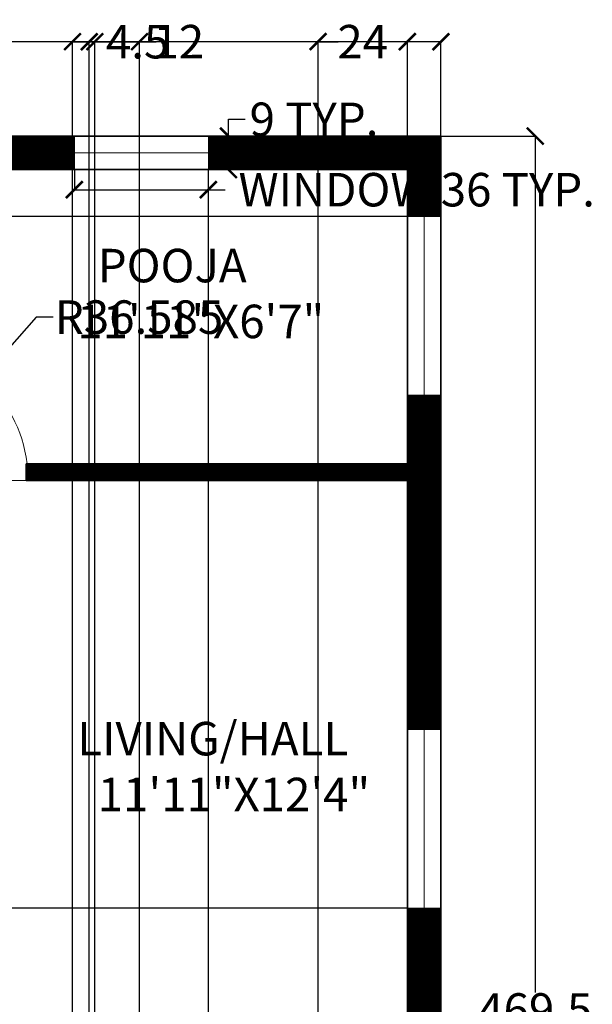
# Model space of a CAD drawing. Units: inches. Extents: x -1 to 426, y -6 to 532.
# Tile 4 of 4: x 228 to 382, y 267 to 532. Entities that reach past the tile are written whole.
import ezdxf

# ---------------------------------------------------------------- set-up
doc = ezdxf.new("R2010")
doc.units = ezdxf.units.IN
doc.header["$MEASUREMENT"] = 0
for name, color, linetype, lineweight in [('A-ANNO-DIMS', 2, 'Continuous', 18), ('A-AREA-IDEN', 7, 'Continuous', 25), ('A-DOOR', 3, 'Continuous', 18), ('A-GLAZ', 4, 'Continuous', 18)]:
    doc.layers.add(name, color=color, linetype=linetype, lineweight=lineweight)
doc.layers.add('A-WALL', color=159, linetype='Continuous', lineweight=35, true_color=0x223569)
doc.layers.add('A-WALL-PATT', color=177, linetype='Continuous', lineweight=13, true_color=0x2c4178)
doc.styles.get("Standard").update_dxf_attribs({"font": 'arial.ttf'})
doc.dimstyles.get("Standard").update_dxf_attribs({"dimtxt": 9, "dimasz": 4.5, "dimexe": 0.18, "dimexo": 0.0625, "dimgap": 0.09, "dimtad": 0, "dimtih": 1, "dimtoh": 1, "dimdec": 1, "dimzin": 0, "dimdsep": 46, "dimlunit": 4, "dimtxsty": 'Standard', "dimblk": 'ARCHTICK', "dimcen": 0.09, "dimadec": 0, "dimazin": 0, "dimtfac": 1, "dimtdec": 1, "dimtofl": 0, "dimtmove": 0, "dimatfit": 3, "dimfxl": 1, "dimtolj": 1, "dimtzin": 0, "dimarcsym": 0})

# ---------------------------------------------------------------- blocks, each defined once
blk = doc.blocks.new('WIN-36IN')
for p, q in [((0, 4.5), (36, 4.5)), ((0, -4.5), (0, 4.5)), ((36, 4.5), (36, -4.5)), ((0, 0), (36, 0)), ((36, -4.5), (0, -4.5))]:
    blk.add_line(p, q)
blk = doc.blocks.new('WIN-48IN')
for p, q in [((-4.5, 48), (4.5, 48)), ((-4.5, 0), (-4.5, 48)), ((0, 48), (0, 0)), ((4.5, 48), (4.5, 0)), ((4.5, 0), (-4.5, 0))]:
    blk.add_line(p, q)
blk = doc.blocks.new('_ArchTick')
at = {"color": 0, "linetype": 'ByBlock', "const_width": 0.15}
blk.add_lwpolyline([(-0.5, -0.5), (0.5, 0.5)], dxfattribs=at)
blk = doc.blocks.new('*D7')
at = {"layer": 'A-ANNO-DIMS', "color": 0, "lineweight": -2, "transparency": 16777216}
for p, q in [((242.32, 491.42), (242.32, 485.9)), ((278.32, 491.42), (278.32, 485.9)), ((242.32, 486.08), (278.32, 486.08)), ((278.32, 486.08), (282.82, 486.08))]:
    blk.add_line(p, q, dxfattribs=at)
at = {"layer": 'Defpoints', "color": 0, "transparency": 16777216}
for p in [(242.32, 491.48), (278.32, 491.48), (278.32, 486.08)]:
    blk.add_point(p, dxfattribs=at)
at = {"layer": 'A-ANNO-DIMS', "color": 0, "lineweight": -2, "transparency": 16777216, "xscale": 4.5, "yscale": 4.5, "zscale": 4.5, "rotation": 180}
blk.add_blockref('_ArchTick', (242.32, 486.08), dxfattribs=at)
at = {"layer": 'A-ANNO-DIMS', "color": 0, "lineweight": -2, "transparency": 16777216, "xscale": 4.5, "yscale": 4.5, "zscale": 4.5}
blk.add_blockref('_ArchTick', (278.32, 486.08), dxfattribs=at)
at = {"layer": 'A-ANNO-DIMS', "color": 0, "transparency": 16777216, "insert": (334.33, 486.08), "char_height": 9, "attachment_point": 5}
blk.add_mtext('\\A1;WINDOW 36 TYP.', dxfattribs=at)
blk = doc.blocks.new('*D8')
at = {"layer": 'A-ANNO-DIMS', "color": 0, "lineweight": -2, "transparency": 16777216}
for p, q in [((283.72, 500.48), (283.72, 504.98)), ((283.72, 504.98), (288.22, 504.98)), ((278.39, 500.48), (283.9, 500.48)), ((283.72, 491.48), (283.72, 500.48)), ((278.39, 491.48), (283.9, 491.48))]:
    blk.add_line(p, q, dxfattribs=at)
at = {"layer": 'Defpoints', "color": 0, "transparency": 16777216}
for p in [(278.32, 500.48), (283.72, 500.48), (278.32, 491.48)]:
    blk.add_point(p, dxfattribs=at)
at = {"layer": 'A-ANNO-DIMS', "color": 0, "lineweight": -2, "transparency": 16777216, "xscale": 4.5, "yscale": 4.5, "zscale": 4.5}
for p, rotation in [((283.72, 500.48), 90), ((283.72, 491.48), 270)]:
    blk.add_blockref('_ArchTick', p, dxfattribs=dict(at, rotation=rotation))
at = {"layer": 'A-ANNO-DIMS', "color": 0, "transparency": 16777216, "insert": (306.72, 504.98), "char_height": 9, "attachment_point": 5}
blk.add_mtext('\\A1;9 TYP.', dxfattribs=at)
blk = doc.blocks.new('*D17')
at = {"layer": 'A-ANNO-DIMS', "color": 0, "lineweight": -2, "transparency": 16777216}
for p, q in [((43.32, 500.54), (43.32, 526.02)), ((43.32, 525.84), (176.69, 525.84)), ((340.82, 525.84), (207.46, 525.84)), ((340.82, 500.54), (340.82, 526.02))]:
    blk.add_line(p, q, dxfattribs=at)
at = {"layer": 'Defpoints', "color": 0, "transparency": 16777216}
for p in [(340.82, 525.84), (43.32, 500.48), (340.82, 500.48)]:
    blk.add_point(p, dxfattribs=at)
at = {"layer": 'A-ANNO-DIMS', "color": 0, "lineweight": -2, "transparency": 16777216, "xscale": 4.5, "yscale": 4.5, "zscale": 4.5, "rotation": 180}
blk.add_blockref('_ArchTick', (43.32, 525.84), dxfattribs=at)
at = {"layer": 'A-ANNO-DIMS', "color": 0, "lineweight": -2, "transparency": 16777216, "xscale": 4.5, "yscale": 4.5, "zscale": 4.5}
blk.add_blockref('_ArchTick', (340.82, 525.84), dxfattribs=at)
at = {"layer": 'A-ANNO-DIMS', "color": 0, "transparency": 16777216, "insert": (192.07, 525.84), "char_height": 9, "attachment_point": 5}
blk.add_mtext('\\A1;297.5', dxfattribs=at)
blk = doc.blocks.new('*D18')
at = {"layer": 'A-ANNO-DIMS', "color": 0, "lineweight": -2, "transparency": 16777216}
for p, q in [((340.89, 500.48), (366.36, 500.48)), ((366.18, 500.48), (366.18, 270.42)), ((366.18, 30.98), (366.18, 261.05)), ((237.39, 30.98), (366.36, 30.98))]:
    blk.add_line(p, q, dxfattribs=at)
at = {"layer": 'Defpoints', "color": 0, "transparency": 16777216}
for p in [(340.82, 500.48), (366.18, 500.48), (237.32, 30.98)]:
    blk.add_point(p, dxfattribs=at)
at = {"layer": 'A-ANNO-DIMS', "color": 0, "lineweight": -2, "transparency": 16777216, "xscale": 4.5, "yscale": 4.5, "zscale": 4.5}
for p, rotation in [((366.18, 500.48), 90), ((366.18, 30.98), 270)]:
    blk.add_blockref('_ArchTick', p, dxfattribs=dict(at, rotation=rotation))
at = {"layer": 'A-ANNO-DIMS', "color": 0, "transparency": 16777216, "insert": (366.18, 265.73), "char_height": 9, "attachment_point": 5}
blk.add_mtext('\\A1;469.5', dxfattribs=at)
blk = doc.blocks.new('*D23')
at = {"layer": 'A-ANNO-DIMS', "color": 0, "lineweight": -2, "transparency": 16777216}
for p, q in [((278.32, 491.42), (278.32, 5.45)), ((331.82, 491.42), (331.82, 5.45)), ((278.32, 5.63), (293.26, 5.63)), ((331.82, 5.63), (316.89, 5.63))]:
    blk.add_line(p, q, dxfattribs=at)
at = {"layer": 'Defpoints', "color": 0, "transparency": 16777216}
for p in [(278.32, 491.48), (331.82, 491.48), (331.82, 5.63)]:
    blk.add_point(p, dxfattribs=at)
at = {"layer": 'A-ANNO-DIMS', "color": 0, "lineweight": -2, "transparency": 16777216, "xscale": 4.5, "yscale": 4.5, "zscale": 4.5, "rotation": 180}
blk.add_blockref('_ArchTick', (278.32, 5.63), dxfattribs=at)
at = {"layer": 'A-ANNO-DIMS', "color": 0, "lineweight": -2, "transparency": 16777216, "xscale": 4.5, "yscale": 4.5, "zscale": 4.5}
blk.add_blockref('_ArchTick', (331.82, 5.63), dxfattribs=at)
at = {"layer": 'A-ANNO-DIMS', "color": 0, "transparency": 16777216, "insert": (305.07, 5.63), "char_height": 9, "attachment_point": 5}
blk.add_mtext('\\A1;53.5', dxfattribs=at)
blk = doc.blocks.new('*D32')
at = {"layer": 'A-ANNO-DIMS', "color": 0, "lineweight": -2, "transparency": 16777216}
for p, q in [((331.76, 293.06), (17.79, 293.06)), ((17.97, 293.06), (17.97, 281.21)), ((17.97, 259.98), (17.97, 271.83)), ((331.76, 259.98), (17.79, 259.98))]:
    blk.add_line(p, q, dxfattribs=at)
at = {"layer": 'Defpoints', "color": 0, "transparency": 16777216}
for p in [(17.97, 293.06), (331.82, 293.06), (331.82, 259.98)]:
    blk.add_point(p, dxfattribs=at)
at = {"layer": 'A-ANNO-DIMS', "color": 0, "lineweight": -2, "transparency": 16777216, "xscale": 4.5, "yscale": 4.5, "zscale": 4.5}
for p, rotation in [((17.97, 293.06), 90), ((17.97, 259.98), 270)]:
    blk.add_blockref('_ArchTick', p, dxfattribs=dict(at, rotation=rotation))
at = {"layer": 'A-ANNO-DIMS', "color": 0, "transparency": 16777216, "insert": (17.97, 276.52), "char_height": 9, "attachment_point": 5}
blk.add_mtext('\\A1;33.08', dxfattribs=at)
blk = doc.blocks.new('*D33')
at = {"layer": 'A-ANNO-DIMS', "color": 0, "lineweight": -2, "transparency": 16777216}
for p, q in [((331.76, 491.48), (17.79, 491.48)), ((17.97, 491.48), (17.97, 489.87)), ((331.76, 478.89), (17.79, 478.89)), ((17.97, 478.89), (17.97, 480.5))]:
    blk.add_line(p, q, dxfattribs=at)
at = {"layer": 'Defpoints', "color": 0, "transparency": 16777216}
for p in [(17.97, 491.48), (331.82, 491.48), (331.82, 478.89)]:
    blk.add_point(p, dxfattribs=at)
at = {"layer": 'A-ANNO-DIMS', "color": 0, "lineweight": -2, "transparency": 16777216, "xscale": 4.5, "yscale": 4.5, "zscale": 4.5}
for p, rotation in [((17.97, 491.48), 90), ((17.97, 478.89), 270)]:
    blk.add_blockref('_ArchTick', p, dxfattribs=dict(at, rotation=rotation))
at = {"layer": 'A-ANNO-DIMS', "color": 0, "transparency": 16777216, "insert": (17.97, 485.19), "char_height": 9, "attachment_point": 5}
blk.add_mtext('\\A1;12.588', dxfattribs=at)
blk = doc.blocks.new('*D35')
at = {"layer": 'A-ANNO-DIMS', "color": 0, "lineweight": -2, "transparency": 16777216}
for p, q in [((247.82, 112.04), (247.82, 526.02)), ((247.82, 525.84), (259.82, 525.84)), ((259.82, 112.04), (259.82, 526.02)), ((259.82, 525.84), (264.32, 525.84))]:
    blk.add_line(p, q, dxfattribs=at)
at = {"layer": 'Defpoints', "color": 0, "transparency": 16777216}
for p in [(259.82, 525.84), (247.82, 111.98), (259.82, 111.98)]:
    blk.add_point(p, dxfattribs=at)
at = {"layer": 'A-ANNO-DIMS', "color": 0, "lineweight": -2, "transparency": 16777216, "xscale": 4.5, "yscale": 4.5, "zscale": 4.5, "rotation": 180}
blk.add_blockref('_ArchTick', (247.82, 525.84), dxfattribs=at)
at = {"layer": 'A-ANNO-DIMS', "color": 0, "lineweight": -2, "transparency": 16777216, "xscale": 4.5, "yscale": 4.5, "zscale": 4.5}
blk.add_blockref('_ArchTick', (259.82, 525.84), dxfattribs=at)
at = {"layer": 'A-ANNO-DIMS', "color": 0, "transparency": 16777216, "insert": (270.39, 525.84), "char_height": 9, "attachment_point": 5}
blk.add_mtext('\\A1;12', dxfattribs=at)
blk = doc.blocks.new('*D38')
at = {"layer": 'A-ANNO-DIMS', "color": 0, "lineweight": -2, "transparency": 16777216}
for p, q in [((307.82, 255.54), (307.82, 526.02)), ((307.82, 525.84), (313.23, 525.84)), ((331.82, 525.84), (326.42, 525.84)), ((331.82, 255.54), (331.82, 526.02))]:
    blk.add_line(p, q, dxfattribs=at)
at = {"layer": 'Defpoints', "color": 0, "transparency": 16777216}
for p in [(331.82, 525.84), (307.82, 255.48), (331.82, 255.48)]:
    blk.add_point(p, dxfattribs=at)
at = {"layer": 'A-ANNO-DIMS', "color": 0, "lineweight": -2, "transparency": 16777216, "xscale": 4.5, "yscale": 4.5, "zscale": 4.5, "rotation": 180}
blk.add_blockref('_ArchTick', (307.82, 525.84), dxfattribs=at)
at = {"layer": 'A-ANNO-DIMS', "color": 0, "lineweight": -2, "transparency": 16777216, "xscale": 4.5, "yscale": 4.5, "zscale": 4.5}
blk.add_blockref('_ArchTick', (331.82, 525.84), dxfattribs=at)
at = {"layer": 'A-ANNO-DIMS', "color": 0, "transparency": 16777216, "insert": (319.82, 525.84), "char_height": 9, "attachment_point": 5}
blk.add_mtext('\\A1;24', dxfattribs=at)
blk = doc.blocks.new('*D46')
at = {"layer": 'A-ANNO-DIMS', "color": 0, "lineweight": -2, "transparency": 16777216}
for p, q in [((241.82, 255.54), (241.82, 526.02)), ((241.82, 525.84), (246.32, 525.84)), ((246.32, 255.54), (246.32, 526.02)), ((246.32, 525.84), (250.82, 525.84))]:
    blk.add_line(p, q, dxfattribs=at)
at = {"layer": 'Defpoints', "color": 0, "transparency": 16777216}
for p in [(246.32, 525.84), (241.82, 255.48), (246.32, 255.48)]:
    blk.add_point(p, dxfattribs=at)
at = {"layer": 'A-ANNO-DIMS', "color": 0, "lineweight": -2, "transparency": 16777216, "xscale": 4.5, "yscale": 4.5, "zscale": 4.5, "rotation": 180}
blk.add_blockref('_ArchTick', (241.82, 525.84), dxfattribs=at)
at = {"layer": 'A-ANNO-DIMS', "color": 0, "lineweight": -2, "transparency": 16777216, "xscale": 4.5, "yscale": 4.5, "zscale": 4.5}
blk.add_blockref('_ArchTick', (246.32, 525.84), dxfattribs=at)
at = {"layer": 'A-ANNO-DIMS', "color": 0, "transparency": 16777216, "insert": (259.32, 525.84), "char_height": 9, "attachment_point": 5}
blk.add_mtext('\\A1;4.5', dxfattribs=at)
blk = doc.blocks.new('*D55')
at = {"layer": 'A-ANNO-DIMS', "color": 0, "lineweight": -2, "transparency": 16777216}
for p, q in [((232.09, 451.85), (217.55, 435.4)), ((236.59, 451.85), (232.09, 451.85)), ((193.23, 407.98), (193.41, 407.98)), ((193.32, 407.89), (193.32, 408.07))]:
    blk.add_line(p, q, dxfattribs=at)
at = {"layer": 'Defpoints', "color": 0, "transparency": 16777216}
for p in [(217.55, 435.4), (193.32, 407.98)]:
    blk.add_point(p, dxfattribs=at)
at = {"layer": 'A-ANNO-DIMS', "color": 0, "lineweight": -2, "transparency": 16777216, "xscale": 4.5, "yscale": 4.5, "zscale": 4.5, "rotation": 228.5330341154112}
blk.add_blockref('_ArchTick', (217.55, 435.4), dxfattribs=at)
at = {"layer": 'A-ANNO-DIMS', "color": 0, "transparency": 16777216, "insert": (259.7, 451.85), "char_height": 9, "attachment_point": 5}
blk.add_mtext('\\A1;R36.585', dxfattribs=at)

msp = doc.modelspace()

# ---------------------------------------------------------------- hatches: boundary and pattern name
at = {"layer": 'A-WALL-PATT'}
h = msp.add_hatch(dxfattribs=at)
h.set_pattern_fill('ANSI31', color=256)
h.set_pattern_definition([(45, (-574.8435, 0), (-0.088388348, 0.088388348), [])])
h.paths.add_polyline_path([(100.3238, 500.4824), (43.3238, 500.4824), (43.3238, 452.5693), (52.3238, 452.5693), (52.3238, 491.4824), (100.3238, 491.4824)])
h.paths.add_polyline_path([(242.3238, 500.4824), (136.3238, 500.4824), (136.3238, 491.4824), (184.3238, 491.4824), (184.3238, 407.9824), (188.8238, 407.9824), (193.3238, 407.9824), (193.3238, 412.4824), (188.8238, 412.4824), (188.8238, 491.4824), (242.3238, 491.4824)])
h.paths.add_polyline_path([(340.8238, 500.4824), (278.3238, 500.4824), (278.3238, 491.4824), (331.8238, 491.4824), (331.8238, 478.8941), (340.8238, 478.8941)])
h.paths.add_polyline_path([(331.8238, 412.4824), (229.3238, 412.4824), (229.3238, 407.9824), (331.8238, 407.9824)])
h.paths.add_polyline_path([(340.8238, 430.8941), (331.8238, 430.8941), (331.8238, 341.0593), (340.8238, 341.0593)])
h.paths.add_polyline_path([(340.8238, 293.0593), (331.8238, 293.0593), (331.8238, 259.9824), (282.3238, 259.9824), (282.3238, 255.4824), (331.8238, 255.4824), (331.8238, 237.2917), (340.8238, 237.2917)])
h.paths.add_polyline_path([(340.8238, 153.5275), (340.8238, 201.2917), (331.8238, 201.2917), (331.8238, 177.4824), (241.8238, 177.4824), (241.8238, 255.4824), (246.3238, 255.4824), (246.3238, 259.9824), (237.3238, 259.9824), (237.3238, 255.4824), (237.3238, 172.9824), (331.8238, 172.9824), (331.8238, 153.5275), (331.8238, 75.9824), (237.3238, 75.9824), (237.3238, 66.9824), (340.8238, 66.9824)])
h.paths.add_polyline_path([(98.5766, 75.9824), (52.3238, 75.9824), (52.3238, 138.3606), (43.3238, 138.3606), (43.3238, 66.9824), (52.3238, 66.9824), (98.5766, 66.9824)])
h.paths.add_polyline_path([(188.8238, 75.9824), (188.8238, 153.5275), (188.8238, 209.4042, -0.02664097), (184.3238, 209.1642), (184.3238, 153.5275), (184.3238, 75.9824), (136.8238, 75.9824), (134.5766, 75.9824), (134.5766, 66.9824), (136.8238, 66.9824), (188.8238, 66.9824)])
h.paths.add_polyline_path([(52.3238, 255.9824), (96.3583, 255.9824), (96.3583, 260.4824), (52.3238, 260.4824), (52.3238, 272.4986), (43.3238, 272.4986), (43.3238, 186.3606), (52.3238, 186.3606)])
h.paths.add_polyline_path([(52.3238, 404.5693), (43.3238, 404.5693), (43.3238, 349.9808), (52.3238, 349.9808), (52.3238, 360.9824), (184.3238, 360.9824), (184.3238, 312.9824), (173.036, 312.9824), (173.036, 308.4824), (184.3238, 308.4824), (188.8238, 308.4824), (188.8238, 365.4824), (184.3238, 365.4824), (52.3238, 365.4824)])
h.paths.add_polyline_path([(188.8238, 260.4824), (136.8238, 260.4824), (136.8238, 308.4824), (136.8238, 312.9824), (52.3238, 312.9824), (52.3238, 332.4824), (43.3238, 332.4824), (43.3238, 308.4824), (43.3238, 296.4986), (52.3238, 296.4986), (52.3238, 298.8674), (52.3238, 308.4824), (132.3238, 308.4824), (132.3238, 260.4824), (132.3238, 255.9824), (136.8238, 255.9824), (184.3238, 255.9824), (184.3238, 251.4824), (186.5738, 251.4824), (188.8238, 251.4824), (188.8238, 255.9824)])

# ---------------------------------------------------------------- linework, layer by layer
at = {"layer": 'A-DOOR'}
msp.add_line((193.3238, 407.9824), (229.3238, 407.9824), dxfattribs=at)
msp.add_arc((193.3238, 407.9824), 36.5854, 7.065274, 90, dxfattribs=at)
at = {"layer": 'A-WALL'}
for p, q in [((43.3238, 500.4824), (340.8238, 500.4824)), ((340.8238, 500.4824), (340.8238, 153.5275)), ((188.8238, 491.4824), (331.8238, 491.4824)), ((331.8238, 491.4824), (331.8238, 259.9824)), ((229.3238, 412.4824), (229.3238, 407.9824)), ((229.3238, 412.4824), (331.8238, 412.4824)), ((229.3238, 407.9824), (331.8238, 407.9824))]:
    msp.add_line(p, q, dxfattribs=at)

# ---------------------------------------------------------------- block references
at = {"layer": 'A-GLAZ'}
for name, p in [('WIN-36IN', (242.3238, 495.9824)), ('WIN-48IN', (336.3238, 430.8941)), ('WIN-48IN', (336.3238, 293.0593))]:
    msp.add_blockref(name, p, dxfattribs=at)

# ---------------------------------------------------------------- texts
at = {"layer": 'A-AREA-IDEN', "char_height": 9, "attachment_point": 1}
for s, insert in [('  POOJA\\P11\'11"X6\'7"', (243.104, 470.1943)), ('LIVING/HALL\\P  11\'11"X12\'4"', (243.104, 343.1215))]:
    msp.add_mtext_dynamic_manual_height_columns(s, width=229.541527, gutter_width=1, heights=[0], dxfattribs=dict(at, insert=insert))

# ---------------------------------------------------------------- dimensions: what is measured, and where the dimension line sits
at = {"layer": 'A-ANNO-DIMS'}
for base, p1, p2, override, picture, middle in [((340.8238, 525.8389), (43.3238, 500.4824), (340.8238, 500.4824), {"dimdec": 1, "dimlfac": 1, "dimrnd": 0, "dimzin": 0, "dimdsep": 46, "dimlunit": 2}, '*D17', (192.0738, 525.8389)), ((246.3238, 525.8389), (241.8238, 255.4824), (246.3238, 255.4824), {"dimdec": 1, "dimlfac": 1, "dimrnd": 0, "dimzin": 0, "dimdsep": 46, "dimlunit": 2}, '*D46', (259.3214, 525.8389)), ((259.8238, 525.8389), (247.8238, 111.9824), (259.8238, 111.9824), {"dimdec": 0, "dimlfac": 1, "dimrnd": 0, "dimzin": 0, "dimdsep": 46, "dimlunit": 2}, '*D35', (270.3902, 525.8389)), ((331.8238, 525.8389), (307.8238, 255.4824), (331.8238, 255.4824), {"dimdec": 0, "dimlfac": 1, "dimrnd": 0, "dimzin": 0, "dimdsep": 46, "dimlunit": 2}, '*D38', (319.8238, 525.8389)), ((331.8238, 5.6259), (278.3238, 491.4824), (331.8238, 491.4824), {"dimdec": 1, "dimlfac": 1, "dimrnd": 0, "dimzin": 0, "dimdsep": 46, "dimlunit": 2}, '*D23', (305.0738, 5.6259))]:
    dim = msp.add_linear_dim(base=base, p1=p1, p2=p2, dimstyle='Standard', override=override, dxfattribs=at)
    dim.commit()
    dim.dimension.update_dxf_attribs({"geometry": picture, "text_midpoint": middle})
dim = msp.add_linear_dim(base=(283.7238, 500.4824), p1=(278.3238, 491.4824), p2=(278.3238, 500.4824), angle=90, text='<> TYP.', dimstyle='Standard', override={"dimdec": 0, "dimlfac": 1, "dimrnd": 0, "dimzin": 0, "dimdsep": 46, "dimlunit": 2}, dxfattribs=at)
dim.commit()
dim.dimension.update_dxf_attribs({"geometry": '*D8', "text_midpoint": (306.722, 504.9824)})
dim = msp.add_linear_dim(base=(278.3238, 486.0824), p1=(242.3238, 491.4824), p2=(278.3238, 491.4824), text='WINDOW <> TYP.', dimstyle='Standard', override={"dimdec": 0, "dimlfac": 1, "dimrnd": 0, "dimzin": 0, "dimdsep": 46, "dimlunit": 2}, dxfattribs=at)
dim.commit()
dim.dimension.update_dxf_attribs({"geometry": '*D7', "text_midpoint": (334.3323, 486.0824)})
for base, p1, p2, override, picture, middle in [((366.1803, 500.4824), (237.3238, 30.9824), (340.8238, 500.4824), {"dimdec": 1, "dimlfac": 1, "dimrnd": 0, "dimzin": 0, "dimdsep": 46, "dimlunit": 2}, '*D18', (366.1803, 265.7324)), ((17.9673, 491.4824), (331.8238, 478.8941), (331.8238, 491.4824), {"dimdec": 3, "dimlfac": 1, "dimrnd": 0, "dimzin": 0, "dimdsep": 46, "dimlunit": 2}, '*D33', (17.9673, 485.1883)), ((17.9673, 293.0593), (331.8238, 259.9824), (331.8238, 293.0593), {"dimdec": 2, "dimlfac": 1, "dimrnd": 0, "dimzin": 0, "dimdsep": 46, "dimlunit": 2}, '*D32', (17.9673, 276.5209))]:
    dim = msp.add_linear_dim(base=base, p1=p1, p2=p2, angle=90, dimstyle='Standard', override=override, dxfattribs=at)
    dim.commit()
    dim.dimension.update_dxf_attribs({"geometry": picture, "text_midpoint": middle})
dim = msp.add_radius_dim(center=(193.3238, 407.9824), mpoint=(217.5502, 435.3972), dimstyle='Standard', override={"dimdec": 3, "dimlfac": 1, "dimrnd": 0, "dimzin": 0, "dimdsep": 46, "dimlunit": 2}, dxfattribs=at)
dim.commit()
dim.dimension.update_dxf_attribs({"geometry": '*D55', "text_midpoint": (259.6978, 451.8461), "dimtype": 164})

doc.saveas('drawing.dxf')
